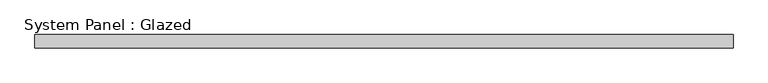
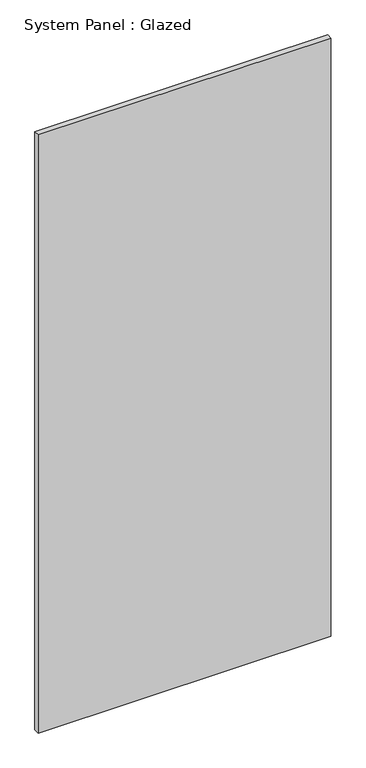
"""IFC4 building model written with IfcOpenShell, lengths in millimetres: plate geometry, System Panel : Glazed."""

from ifc_helpers import new_model, si_unit, origin, origin_with_axes, place, context, project, spatial, polyline, outline, extrude, source, transform, mapped, element, save


def system_panel_glazed_f623c012(model_context):
    return source(origin(), model_context, "Body", "SweptSolid", [
        extrude(outline(polyline([(675.8408525, 19.05), (-675.8408525, 19.05), (-675.8408525, 44.45), (675.8408525, 44.45), (675.8408525, 19.05)])), origin_with_axes(), (0.0, 0.0, 1.0), 2921.0),
    ])


if __name__ == "__main__":
    model = new_model("IFC4")
    model_context = context("Model", 3, world=origin())
    ifc_project = project(units=[si_unit("LENGTHUNIT", "METRE", prefix="MILLI")], contexts=[model_context])
    site = spatial("IfcSite", under=ifc_project)
    building = spatial("IfcBuilding", under=site)
    placement = place(None, origin())
    system_panel_glazed_shape = system_panel_glazed_f623c012(model_context)
    element("IfcPlate", 1, ObjectType="System Panel : Glazed", at=placement, inside=building, context=model_context, shape_type="MappedRepresentation", body=[
        mapped(system_panel_glazed_shape, transform((0.0, 0.0, 0.0), x_axis=(1.0, 0.0, 0.0), y_axis=(0.0, 1.0, 0.0), z_axis=(0.0, 0.0, 1.0))),
    ])
    save(model, "model.ifc")

# Revit data of these elements
# Type "System Panel : Glazed"
#   Construction Type Id = "GSP4R"
#   Analytic Construction = "1/8 in Pilkington single glazing"
#   Visual Light Transmittance = 0.9
#   Solar Heat Gain Coefficient = 0.86
#   Heat Transfer Coefficient (U) = 1.18115 BTU/(h·ft²·°F)
# Element 1 (IfcPlate, "System Panel : Glazed")
#   Materials on its faces: "Glass"
# Materials
#   "Glass": class "Glass", colour RGB 0 128 192, transparency 0.75, Description = "Soda Lime Glass", Cost = 0
